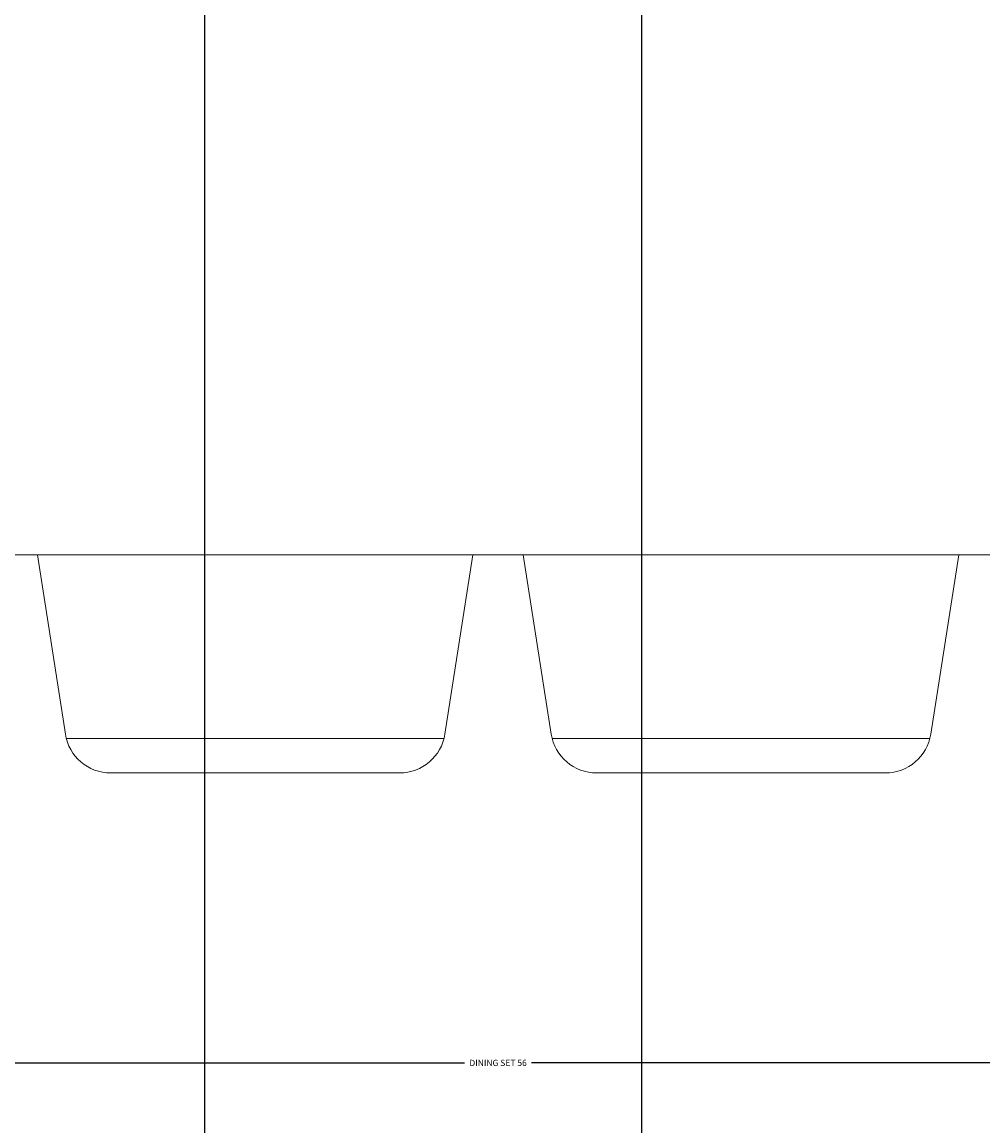
# Model space of a CAD drawing. Units: inches. Extents: x 2231 to 2461, y 2045 to 2455.
# Tile 24 of 95: x 2343 to 2371, y 2112 to 2144. Entities that reach past the tile are written whole.
import ezdxf

# ---------------------------------------------------------------- set-up
doc = ezdxf.new("R2010")
doc.units = ezdxf.units.IN
doc.layers.add('A-ANNO-DIMS', color=2, linetype='Continuous', lineweight=18)
doc.layers.add('A-FURN', color=9, linetype='Continuous', lineweight=18)
doc.styles.get("Standard").update_dxf_attribs({"font": 'arial.ttf'})
doc.dimstyles.get("Standard").update_dxf_attribs({"dimtxt": 0.18, "dimasz": 0.18, "dimexe": 0.18, "dimexo": 0.0625, "dimgap": 0.09, "dimtad": 0, "dimtih": 1, "dimtoh": 1, "dimdec": 4, "dimzin": 0, "dimdsep": 46, "dimtxsty": 'Standard', "dimcen": 0.09, "dimadec": 0, "dimazin": 0, "dimtfac": 1, "dimtdec": 4, "dimtofl": 0, "dimtmove": 0, "dimatfit": 3, "dimfxl": 1, "dimtolj": 1, "dimtzin": 0, "dimarcsym": 0})

# ---------------------------------------------------------------- blocks, each defined once
blk = doc.blocks.new('Dining Set - 36 x 72 in.')
for p, q in [((-36, -18), (-4.062, -18)), ((-22.264, -25.809), (-23.485, -17.998)), ((-4.515, -17.998), (-5.736, -25.809)), ((-4.062, -18), (29.162, -18)), ((-1.102, -25.809), (-2.322, -17.998)), ((16.647, -17.998), (15.427, -25.809)), ((-22.23, -26), (-5.761, -26)), ((-1.068, -26), (15.402, -26)), ((-20.288, -27.5), (-7.712, -27.5)), ((0.874, -27.5), (13.451, -27.5))]:
    blk.add_line(p, q)
for centre, start, end in [((-20.288, -25.5), 188.8802, 270), ((-7.712, -25.5), 270, 351.1191), ((0.874, -25.5), 188.8802, 270), ((13.451, -25.5), 270, 351.1191)]:
    blk.add_arc(centre, 2, start, end)
blk = doc.blocks.new('*D31')
at = {"layer": 'A-ANNO-DIMS', "color": 0, "lineweight": -2, "transparency": 16777216}
for p, q in [((2328.765, 2122.602), (2328.765, 2114.118)), ((2384.543, 2122.602), (2384.543, 2114.118)), ((2328.945, 2114.298), (2355.685, 2114.298)), ((2384.363, 2114.298), (2357.623, 2114.298))]:
    blk.add_line(p, q, dxfattribs=at)
at = {"layer": 'A-ANNO-DIMS', "color": 0, "transparency": 16777216}
for points in [[(2328.945, 2114.328), (2328.945, 2114.268), (2328.765, 2114.298)], [(2384.363, 2114.328), (2384.363, 2114.268), (2384.543, 2114.298)]]:
    blk.add_solid(points, dxfattribs=at)
at = {"layer": 'Defpoints', "color": 0, "transparency": 16777216}
for p in [(2328.765, 2122.665), (2384.543, 2122.665), (2384.543, 2114.298)]:
    blk.add_point(p, dxfattribs=at)
at = {"layer": 'A-ANNO-DIMS', "color": 0, "transparency": 16777216, "insert": (2356.654, 2114.298), "char_height": 0.18, "attachment_point": 5}
blk.add_mtext('\\A1;DINING SET 56', dxfattribs=at)
blk = doc.blocks.new('*D52')
at = {"layer": 'A-ANNO-DIMS', "color": 0, "lineweight": -2, "transparency": 16777216}
for p, q in [((2330.794, 2306.77), (2330.794, 2044.803)), ((2360.794, 2306.77), (2360.794, 2044.803)), ((2330.974, 2044.983), (2345.575, 2044.983)), ((2360.614, 2044.983), (2346.012, 2044.983))]:
    blk.add_line(p, q, dxfattribs=at)
at = {"layer": 'A-ANNO-DIMS', "color": 0, "transparency": 16777216}
for points in [[(2330.974, 2045.013), (2330.974, 2044.953), (2330.794, 2044.983)], [(2360.614, 2045.013), (2360.614, 2044.953), (2360.794, 2044.983)]]:
    blk.add_solid(points, dxfattribs=at)
at = {"layer": 'Defpoints', "color": 0, "transparency": 16777216}
for p in [(2330.794, 2306.833), (2360.794, 2306.833), (2360.794, 2044.983)]:
    blk.add_point(p, dxfattribs=at)
at = {"layer": 'A-ANNO-DIMS', "color": 0, "transparency": 16777216, "insert": (2345.794, 2044.983), "char_height": 0.18, "attachment_point": 5}
blk.add_mtext('\\A1;30', dxfattribs=at)
blk = doc.blocks.new('*D66')
at = {"layer": 'A-ANNO-DIMS', "color": 0, "lineweight": -2, "transparency": 16777216}
for p, q in [((2348.189, 2096.895), (2348.189, 2454.645)), ((2348.369, 2454.465), (2378.167, 2454.465)), ((2408.614, 2454.465), (2378.815, 2454.465)), ((2408.794, 2096.895), (2408.794, 2454.645))]:
    blk.add_line(p, q, dxfattribs=at)
at = {"layer": 'A-ANNO-DIMS', "color": 0, "transparency": 16777216}
for points in [[(2348.369, 2454.495), (2348.369, 2454.435), (2348.189, 2454.465)], [(2408.614, 2454.495), (2408.614, 2454.435), (2408.794, 2454.465)]]:
    blk.add_solid(points, dxfattribs=at)
at = {"layer": 'Defpoints', "color": 0, "transparency": 16777216}
for p in [(2408.794, 2454.465), (2348.189, 2096.833), (2408.794, 2096.833)]:
    blk.add_point(p, dxfattribs=at)
at = {"layer": 'A-ANNO-DIMS', "color": 0, "transparency": 16777216, "insert": (2378.491, 2454.465), "char_height": 0.18, "attachment_point": 5}
blk.add_mtext('\\A1;60.6', dxfattribs=at)
blk = doc.blocks.new('*D69')
at = {"layer": 'A-ANNO-DIMS', "color": 0, "lineweight": -2, "transparency": 16777216}
for p, q in [((2340.667, 2189.285), (2340.667, 2044.803)), ((2394.794, 2186.77), (2394.794, 2044.803)), ((2340.847, 2044.983), (2367.337, 2044.983)), ((2394.614, 2044.983), (2368.124, 2044.983))]:
    blk.add_line(p, q, dxfattribs=at)
at = {"layer": 'A-ANNO-DIMS', "color": 0, "transparency": 16777216}
for points in [[(2340.847, 2045.013), (2340.847, 2044.953), (2340.667, 2044.983)], [(2394.614, 2045.013), (2394.614, 2044.953), (2394.794, 2044.983)]]:
    blk.add_solid(points, dxfattribs=at)
at = {"layer": 'Defpoints', "color": 0, "transparency": 16777216}
for p in [(2340.667, 2189.348), (2394.794, 2186.833), (2394.794, 2044.983)]:
    blk.add_point(p, dxfattribs=at)
at = {"layer": 'A-ANNO-DIMS', "color": 0, "transparency": 16777216, "insert": (2367.73, 2044.983), "char_height": 0.18, "attachment_point": 5}
blk.add_mtext('\\A1;54.13', dxfattribs=at)

msp = doc.modelspace()

# ---------------------------------------------------------------- block references
at = {"layer": 'A-FURN', "xscale": 0.6627357546055535, "yscale": 0.6627357546055535, "zscale": 0.6627357546055535}
msp.add_blockref('Dining Set - 36 x 72 in.', (2358.9199, 2140.8902), dxfattribs=at)

# ---------------------------------------------------------------- dimensions: what is measured, and where the dimension line sits
at = {"layer": 'A-ANNO-DIMS'}
for base, p1, p2, override, picture, middle in [((2408.7935, 2454.4653), (2348.1888, 2096.8328), (2408.7935, 2096.8328), {"dimdec": 1, "dimlfac": 1, "dimrnd": 0, "dimzin": 0, "dimdsep": 46, "dimlunit": 2}, '*D66', (2378.4912, 2454.4653)), ((2360.7935, 2044.9825), (2330.7935, 2306.8328), (2360.7935, 2306.8328), {"dimdec": 0, "dimlfac": 1, "dimrnd": 0, "dimzin": 0, "dimdsep": 46, "dimlunit": 2}, '*D52', (2345.7935, 2044.9825)), ((2394.7935, 2044.9825), (2340.6673, 2189.3477), (2394.7935, 2186.8328), {"dimdec": 2, "dimlfac": 1, "dimrnd": 0, "dimzin": 0, "dimdsep": 46, "dimlunit": 2}, '*D69', (2367.7304, 2044.9825))]:
    dim = msp.add_linear_dim(base=base, p1=p1, p2=p2, dimstyle='Standard', override=override, dxfattribs=at)
    dim.commit()
    dim.dimension.update_dxf_attribs({"geometry": picture, "text_midpoint": middle})
dim = msp.add_linear_dim(base=(2384.5428, 2114.2984), p1=(2328.7655, 2122.665), p2=(2384.5428, 2122.665), text='DINING SET <>', dimstyle='Standard', override={"dimdec": 0, "dimlfac": 1, "dimrnd": 0, "dimzin": 0, "dimdsep": 46, "dimlunit": 2}, dxfattribs=at)
dim.commit()
dim.dimension.update_dxf_attribs({"geometry": '*D31', "text_midpoint": (2356.6542, 2114.2984)})

doc.saveas('drawing.dxf')
